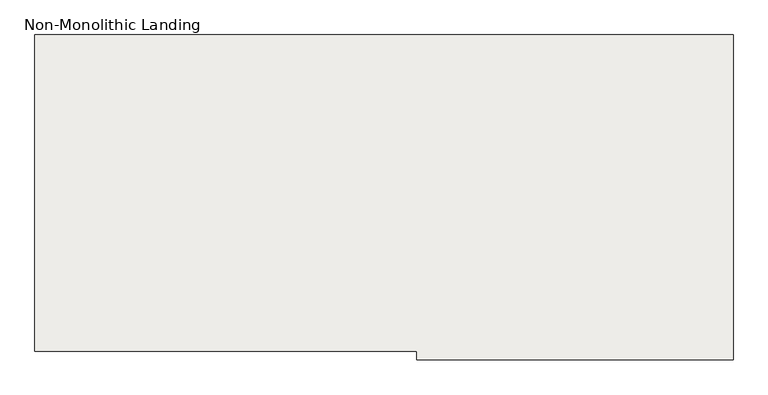
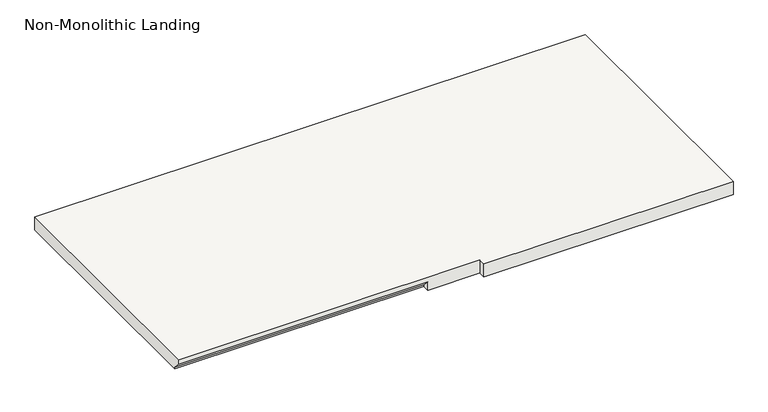
"""IFC4 building model written with IfcOpenShell, lengths in millimetres: slab geometry, Non-Monolithic Landing."""

from ifc_helpers import new_model, si_unit, origin, place, context, project, spatial, faceted_brep, source, transform, mapped, element, save


def non_monolithic_landing_e0ece5e3(model_context):
    return source(origin(), model_context, "Body", "Brep", [
        faceted_brep([(-12643.368339, 8412.443496, 5391.15), (-12643.368339, 8437.843496, 5365.75), (-11728.968339, 8437.843496, 5365.75), (-11728.968339, 8412.443496, 5391.15), (-11538.468339, 8412.443496, 5410.2), (-11538.468339, 8387.043496, 5410.2), (-10624.068339, 8387.043496, 5410.2), (-10624.068339, 8412.443496, 5410.2), (-10624.068339, 9326.843496, 5410.2), (-12643.368339, 9326.843496, 5410.2), (-12643.368339, 8412.443496, 5410.2), (-11728.968339, 8437.843496, 5359.4), (-12643.368339, 8437.843496, 5359.4), (-12643.368339, 9326.843496, 5359.4), (-10624.068339, 9326.843496, 5359.4), (-10624.068339, 8412.443496, 5359.4), (-10624.068339, 8387.043496, 5359.4), (-11538.468339, 8387.043496, 5359.4), (-11538.468339, 8412.443496, 5359.4), (-11728.968339, 8412.443496, 5359.4)], [[[0, 1, 2, 3]], [[4, 5, 6, 7, 8, 9, 10]], [[11, 12, 13, 14, 15, 16, 17, 18, 19]], [[12, 11, 2, 1]], [[11, 19, 3, 2]], [[4, 10, 0, 3, 19, 18]], [[5, 4, 18, 17]], [[6, 5, 17, 16]], [[7, 6, 16, 15]], [[8, 7, 15, 14]], [[9, 8, 14, 13]], [[10, 9, 13, 12, 1, 0]]]),
    ])


if __name__ == "__main__":
    model = new_model("IFC4")
    model_context = context("Model", 3, world=origin())
    ifc_project = project(units=[si_unit("LENGTHUNIT", "METRE", prefix="MILLI")], contexts=[model_context])
    site = spatial("IfcSite", under=ifc_project)
    building = spatial("IfcBuilding", under=site)
    placement = place(None, origin())
    non_monolithic_landing_shape = non_monolithic_landing_e0ece5e3(model_context)
    element("IfcSlab", 1, ObjectType="Non-Monolithic Landing", at=placement, inside=building, context=model_context, shape_type="MappedRepresentation", body=[
        mapped(non_monolithic_landing_shape, transform((0.0, 0.0, 0.0), x_axis=(1.0, 0.0, 0.0), y_axis=(0.0, 1.0, 0.0), z_axis=(0.0, 0.0, 1.0))),
    ])
    save(model, "model.ifc")
